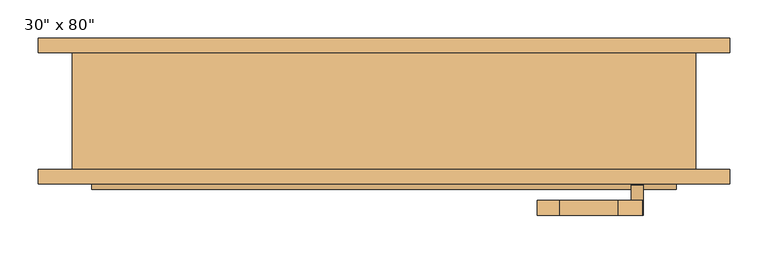
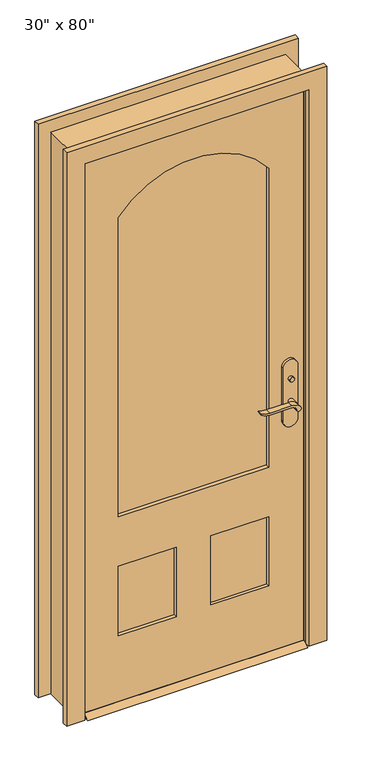
"""IFC4 building model written with IfcOpenShell, lengths in millimetres: door geometry."""

from ifc_helpers import new_model, si_unit, point, frame, frame_2d, origin, place, context, project, spatial, polyline, circle_curve, trimmed, segment, composite_curve, outline, extrude, faceted_brep, source, transform, mapped, element, save


def door_4b146b56(model_context):
    return source(origin(), model_context, "Body", "SolidModel", [
        extrude(outline(polyline([(-38.1, 12.7), (-12.7, 0.0), (-98.425, 0.0), (-73.025, 12.7), (-38.1, 12.7)])), frame((-381.0, 0.0, 0.0), z_axis=(1.0, 0.0, 0.0), x_axis=(0.0, 1.0, 0.0)), (0.0, 0.0, 1.0), 762.0),
        extrude(outline(polyline([(335.2, -18.1), (335.2, -28.1), (325.2, -28.1), (325.2, -18.1), (335.2, -18.1)])), frame((0.0, 0.0, 981.9), z_axis=(0.0, 0.0, 1.0), x_axis=(1.0, 0.0, 0.0)), (0.0, 0.0, 1.0), 30.0),
        extrude(outline(composite_curve([segment(trimmed(circle_curve(frame_2d((996.9, 330.2)), 8.0), [point((996.9, 322.2))], [point((996.9, 338.2))], False, "CARTESIAN"), True, "CONTINUOUS"), segment(trimmed(circle_curve(frame_2d((996.9, 330.2)), 8.0), [point((996.9, 338.2))], [point((996.9, 322.2))], False, "CARTESIAN"), True, "CONTINUOUS")], self_intersect=False)), frame((0.0, -93.025, 0.0), z_axis=(0.0, 1.0, 0.0), x_axis=(0.0, 0.0, 1.0)), (0.0, 0.0, 1.0), 10.0),
        extrude(outline(composite_curve([segment(trimmed(circle_curve(frame_2d((897.1555521, 306.5324871)), 37.2832219), [point((919.0523287, 336.7081363))], [point((934.4, 304.8325667))], False, "CARTESIAN"), True, "CONTINUOUS"), segment(polyline([(934.4, 304.8325667), (934.4, 228.5564091)]), True, "CONTINUOUS"), segment(trimmed(circle_curve(frame_2d((1017.6850638, 228.6227909)), 83.2850902), [point((934.4, 228.5564091))], [point((939.4, 200.2))], True, "CARTESIAN"), True, "CONTINUOUS"), segment(polyline([(939.4, 200.2), (936.6135558, 200.2)]), True, "CONTINUOUS"), segment(trimmed(circle_curve(frame_2d((986.6709207, 232.1396612)), 59.3791355), [point((936.6135558, 200.2))], [point((927.4, 228.5564091))], False, "CARTESIAN"), True, "CONTINUOUS"), segment(polyline([(927.4, 228.5564091), (927.4, 304.8138099)]), True, "CONTINUOUS"), segment(trimmed(circle_curve(frame_2d((909.2738613, 304.8138099)), 18.1261387), [point((927.4, 304.8138099))], [point((914.4, 322.2))], True, "CARTESIAN"), True, "CONTINUOUS"), segment(trimmed(circle_curve(frame_2d((914.4, 330.2)), 8.0), [point((914.4, 322.2))], [point((919.0523287, 336.7081363))], False, "CARTESIAN"), True, "CONTINUOUS")], self_intersect=False)), frame((0.0, 1.9, 0.0), z_axis=(0.0, 1.0, 0.0), x_axis=(0.0, 0.0, 1.0)), (0.0, 0.0, 1.0), 20.0),
        extrude(outline(composite_curve([segment(trimmed(circle_curve(frame_2d((914.4, 330.2)), 8.0), [point((914.3999903, 322.2))], [point((919.0523287, 336.7081363))], False, "CARTESIAN"), True, "CONTINUOUS"), segment(trimmed(circle_curve(frame_2d((897.1555521, 306.5324871)), 37.2832219), [point((919.0523287, 336.7081363))], [point((934.4, 304.8325667))], False, "CARTESIAN"), True, "CONTINUOUS"), segment(polyline([(934.4, 304.8325667), (934.4, 228.5564091)]), True, "CONTINUOUS"), segment(trimmed(circle_curve(frame_2d((1017.6850638, 228.6227909)), 83.2850902), [point((934.4, 228.5564091))], [point((939.4, 200.2))], True, "CARTESIAN"), True, "CONTINUOUS"), segment(polyline([(939.4, 200.2), (936.6135558, 200.2)]), True, "CONTINUOUS"), segment(trimmed(circle_curve(frame_2d((986.6709207, 232.1396612)), 59.3791355), [point((936.6135558, 200.2))], [point((927.4, 228.5564091))], False, "CARTESIAN"), True, "CONTINUOUS"), segment(polyline([(927.4, 228.5564091), (927.4, 304.8138122)]), True, "CONTINUOUS"), segment(trimmed(circle_curve(frame_2d((909.2738682, 304.8138122)), 18.1261318), [point((927.4, 304.8138122))], [point((914.3999903, 322.2))], True, "CARTESIAN"), True, "CONTINUOUS")], self_intersect=False)), frame((0.0, -133.025, 0.0), z_axis=(0.0, 1.0, 0.0), x_axis=(0.0, 0.0, 1.0)), (0.0, 0.0, 1.0), 20.0),
        extrude(outline(composite_curve([segment(trimmed(circle_curve(frame_2d((914.4, 330.2)), 8.0), [point((914.4, 322.2))], [point((914.4, 338.2))], False, "CARTESIAN"), True, "CONTINUOUS"), segment(trimmed(circle_curve(frame_2d((914.4, 330.2)), 8.0), [point((914.4, 338.2))], [point((914.4, 322.2))], False, "CARTESIAN"), True, "CONTINUOUS")], self_intersect=False)), frame((0.0, -28.1, 0.0), z_axis=(0.0, 1.0, 0.0), x_axis=(0.0, 0.0, 1.0)), (0.0, 0.0, 1.0), 30.0),
        extrude(outline(composite_curve([segment(trimmed(circle_curve(frame_2d((914.4, 330.2)), 8.0), [point((914.4, 322.2))], [point((914.4, 338.2))], False, "CARTESIAN"), True, "CONTINUOUS"), segment(trimmed(circle_curve(frame_2d((914.4, 330.2)), 8.0), [point((914.4, 338.2))], [point((914.4, 322.2))], False, "CARTESIAN"), True, "CONTINUOUS")], self_intersect=False)), frame((0.0, -113.025, 0.0), z_axis=(0.0, 1.0, 0.0), x_axis=(0.0, 0.0, 1.0)), (0.0, 0.0, 1.0), 30.0),
        extrude(outline(composite_curve([segment(polyline([(844.4, 355.2), (1039.4, 355.2)]), True, "CONTINUOUS"), segment(trimmed(circle_curve(frame_2d((1039.4, 330.2)), 25.0), [point((1039.4, 355.2))], [point((1039.4, 305.2))], False, "CARTESIAN"), True, "CONTINUOUS"), segment(polyline([(1039.4, 305.2), (844.4, 305.2)]), True, "CONTINUOUS"), segment(trimmed(circle_curve(frame_2d((844.4, 330.2)), 25.0), [point((844.4, 305.2))], [point((844.4, 355.2))], False, "CARTESIAN"), True, "CONTINUOUS")], self_intersect=False)), frame((0.0, -38.1, 0.0), z_axis=(0.0, 1.0, 0.0), x_axis=(0.0, 0.0, 1.0)), (0.0, 0.0, 1.0), 10.0),
        extrude(outline(composite_curve([segment(polyline([(844.4, 355.2), (1039.4, 355.2)]), True, "CONTINUOUS"), segment(trimmed(circle_curve(frame_2d((1039.4, 330.2)), 25.0), [point((1039.4, 355.2))], [point((1039.4, 305.2))], False, "CARTESIAN"), True, "CONTINUOUS"), segment(polyline([(1039.4, 305.2), (844.4, 305.2)]), True, "CONTINUOUS"), segment(trimmed(circle_curve(frame_2d((844.4, 330.2)), 25.0), [point((844.4, 305.2))], [point((844.4, 355.2))], False, "CARTESIAN"), True, "CONTINUOUS")], self_intersect=False)), frame((0.0, -83.025, 0.0), z_axis=(0.0, 1.0, 0.0), x_axis=(0.0, 0.0, 1.0)), (0.0, 0.0, 1.0), 10.0),
        extrude(outline(polyline([(2032.0, -381.0), (12.7, -381.0), (12.7, 381.0), (2032.0, 381.0), (2032.0, -381.0)]), holes=[composite_curve([segment(polyline([(688.975, -260.35), (1784.35, -260.35)]), True, "CONTINUOUS"), segment(trimmed(circle_curve(frame_2d((1580.99125, 0.0)), 330.35875), [point((1784.35, -260.35))], [point((1784.35, 260.35))], True, "CARTESIAN"), True, "CONTINUOUS"), segment(polyline([(1784.35, 260.35), (688.975, 260.35), (688.975, -260.35)]), True, "CONTINUOUS")], self_intersect=False), polyline([(508.0, -60.325), (254.0, -60.325), (254.0, -260.35), (508.0, -260.35), (508.0, -60.325)]), polyline([(508.0, 260.35), (254.0, 260.35), (254.0, 60.325), (508.0, 60.325), (508.0, 260.35)])]), frame((0.0, -73.025, 0.0), z_axis=(0.0, 1.0, 0.0), x_axis=(0.0, 0.0, 1.0)), (0.0, 0.0, 1.0), 34.925),
        faceted_brep([(406.4, -73.025, 0.0), (381.0, -73.025, 0.0), (381.0, -38.1, 0.0), (368.3, -38.1, 0.0), (368.3, -3.175, 0.0), (381.0, -3.175, 0.0), (381.0, 79.375, 0.0), (406.4, 79.375, 0.0), (406.4, 79.375, 2057.4), (406.4, -73.025, 2057.4), (381.0, 79.375, 2032.0), (-381.0, 79.375, 2032.0), (-381.0, 79.375, 0.0), (-406.4, 79.375, 0.0), (-406.4, 79.375, 2057.4), (381.0, -3.175, 2032.0), (368.3, -3.175, 2019.3), (-368.3, -3.175, 2019.3), (-368.3, -3.175, 0.0), (-381.0, -3.175, 0.0), (-381.0, -3.175, 2032.0), (368.3, -38.1, 2019.3), (381.0, -38.1, 2032.0), (-381.0, -38.1, 2032.0), (-381.0, -38.1, 0.0), (-368.3, -38.1, 0.0), (-368.3, -38.1, 2019.3), (381.0, -73.025, 2032.0), (-406.4, -73.025, 2057.4), (-406.4, -73.025, 0.0), (-381.0, -73.025, 0.0), (-381.0, -73.025, 2032.0)], [[[0, 1, 2, 3, 4, 5, 6, 7]], [[7, 8, 9, 0]], [[6, 10, 11, 12, 13, 14, 8, 7]], [[5, 15, 10, 6]], [[4, 16, 17, 18, 19, 20, 15, 5]], [[3, 21, 16, 4]], [[2, 22, 23, 24, 25, 26, 21, 3]], [[1, 27, 22, 2]], [[0, 9, 28, 29, 30, 31, 27, 1]], [[8, 14, 28, 9]], [[15, 20, 11, 10]], [[21, 26, 17, 16]], [[27, 31, 23, 22]], [[29, 13, 12, 19, 18, 25, 24, 30]], [[14, 13, 29, 28]], [[20, 19, 12, 11]], [[26, 25, 18, 17]], [[31, 30, 24, 23]]]),
        extrude(outline(polyline([(-60.325, -49.7416667), (-60.325, -61.3833333), (-260.35, -61.3833333), (-260.35, -49.7416667), (-60.325, -49.7416667)])), frame((0.0, 0.0, 254.0), z_axis=(0.0, 0.0, 1.0), x_axis=(1.0, 0.0, 0.0)), (0.0, 0.0, 1.0), 254.0),
        extrude(outline(polyline([(260.35, -49.7416667), (260.35, -61.3833333), (60.325, -61.3833333), (60.325, -49.7416667), (260.35, -49.7416667)])), frame((0.0, 0.0, 254.0), z_axis=(0.0, 0.0, 1.0), x_axis=(1.0, 0.0, 0.0)), (0.0, 0.0, 1.0), 254.0),
        extrude(outline(composite_curve([segment(polyline([(688.975, -260.35), (688.975, 260.35), (1784.35, 260.35)]), True, "CONTINUOUS"), segment(trimmed(circle_curve(frame_2d((1580.99125, 0.0)), 330.35875), [point((1784.35, 260.35))], [point((1784.35, -260.35))], False, "CARTESIAN"), True, "CONTINUOUS"), segment(polyline([(1784.35, -260.35), (688.975, -260.35)]), True, "CONTINUOUS")], self_intersect=False)), frame((0.0, -59.055, 0.0), z_axis=(0.0, 1.0, 0.0), x_axis=(0.0, 0.0, 1.0)), (0.0, 0.0, 1.0), 6.985),
        extrude(outline(polyline([(0.0, -387.35), (2038.35, -387.35), (2038.35, 387.35), (0.0, 387.35), (0.0, 450.85), (2101.85, 450.85), (2101.85, -450.85), (0.0, -450.85), (0.0, -387.35)])), frame((0.0, 79.375, 0.0), z_axis=(0.0, 1.0, 0.0), x_axis=(0.0, 0.0, 1.0)), (0.0, 0.0, 1.0), 19.05),
        extrude(outline(polyline([(0.0, -387.35), (2038.35, -387.35), (2038.35, 387.35), (0.0, 387.35), (0.0, 450.85), (2101.85, 450.85), (2101.85, -450.85), (0.0, -450.85), (0.0, -387.35)])), frame((0.0, -92.075, 0.0), z_axis=(0.0, 1.0, 0.0), x_axis=(0.0, 0.0, 1.0)), (0.0, 0.0, 1.0), 19.05),
    ])


if __name__ == "__main__":
    model = new_model("IFC4")
    model_context = context("Model", 3, world=origin())
    ifc_project = project(units=[si_unit("LENGTHUNIT", "METRE", prefix="MILLI")], contexts=[model_context])
    site = spatial("IfcSite", under=ifc_project)
    building = spatial("IfcBuilding", under=site)
    placement = place(None, origin())
    door_shape = door_4b146b56(model_context)
    element("IfcDoor", 1, ObjectType="30\" x 80\"", at=placement, inside=building, context=model_context, shape_type="MappedRepresentation", body=[
        mapped(door_shape, transform((0.0, 0.0, 0.0), x_axis=(1.0, 0.0, 0.0), y_axis=(0.0, 1.0, 0.0), z_axis=(0.0, 0.0, 1.0))),
    ])
    save(model, "model.ifc")

# Revit data of these elements
# Type "30\" x 80\""
#   Type Mark = "8"
#   Assembly Code = "B2030100"
#   Analytic Construction = "French door, wood frame with single glass"
#   Threshold Offset [instance default] = 0' - 0 1/2"
#   Thickness = 0' - 1 3/8"
#   Thermal Resistance (R) = 1.0696 (h·ft²·°F)/BTU
#   Swing Angle [instance default] = 90.00°
#   Stiles = 0' - 4 3/4"
#   Rough Width = 2' - 8"
#   Rough Height = 6' - 9"
#   Radius = 1' - 1.00625"
#   Lock Rail = 0' - 7 1/8"
#   Height = 6' - 8"
#   Width = 2' - 6"
#   Heat Transfer Coefficient (U) = 0.9350 BTU/(h·ft²·°F)
#   Door Offset [instance default] = 0' - 0"
#   Bottom Rail = 0' - 9 1/2"
#   Threshold [instance default] = yes
#   Function = 1
#   Exterior Trim [instance default] = yes
#   Trim Material = Cherry
#   Threshold Material = Cherry
#   Panel Material = Cherry
#   Glazing = Glass
#   Frame Material = Cherry
#   Door Handle Material = Aluminum
#   Visual Light Transmittance = 0
#   Solar Heat Gain Coefficient = 0
#   Wall Closure = (empty or 0)
#   Construction Type = (empty or 0)
# Element 1 (IfcDoor, "30\" x 80\"")
#   Materials on its faces: "Cherry", "Aluminum", "Glass"
# Materials
#   "Cherry": class "Wood", colour RGB 226 177 128, transparency 0, Description = "Prunus Serotina", Cost = 0
#   "Glass": class "Glass", colour RGB 0 128 192, transparency 0.75, Description = "Soda Lime Glass", Cost = 0
#   "Aluminum": class "Metal", colour RGB 247 247 247, transparency 0, Description = "Aluminum 6061", Cost = 0
